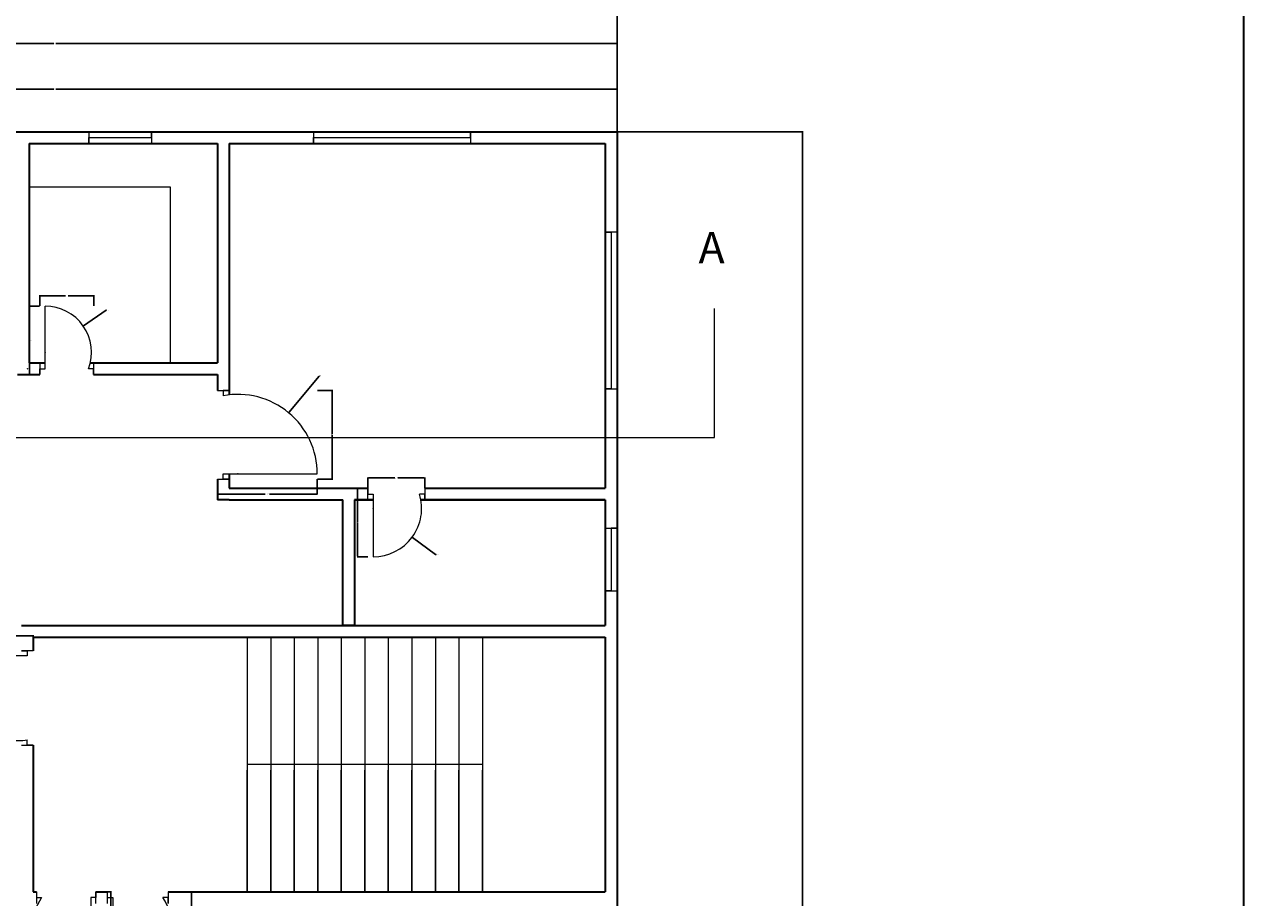
# Model space of a CAD drawing. Units: inches. Extents: x 992 to 2287, y 1476 to 2866.
# Tile 7 of 9: x 1821 to 2287, y 1987 to 2321. Entities that reach past the tile are written whole.
import ezdxf

# ---------------------------------------------------------------- set-up
doc = ezdxf.new("R2010")
doc.units = ezdxf.units.IN
for name, color, linetype, lineweight in [('A-ANNO-DIMS', 2, 'Continuous', 18), ('A-ANNO-SYMB', 2, 'Continuous', 18), ('A-ANNO-TTLB', 7, 'Continuous', 35), ('A-DOOR', 3, 'Continuous', 18), ('A-FLOR-CASE', 9, 'Continuous', 18), ('A-FLOR-STRS', 7, 'Continuous', 18), ('A-GLAZ', 4, 'Continuous', 18), ('A-WALL', 7, 'Continuous', 35)]:
    doc.layers.add(name, color=color, linetype=linetype, lineweight=lineweight)
doc.styles.get("Standard").update_dxf_attribs({"font": 'arial.ttf'})
doc.dimstyles.get("Standard").update_dxf_attribs({"dimtxt": 0.18, "dimasz": 0.18, "dimexe": 0.18, "dimexo": 0.0625, "dimgap": 0.09, "dimtad": 0, "dimtih": 1, "dimtoh": 1, "dimdec": 4, "dimzin": 0, "dimdsep": 46, "dimtxsty": 'Standard', "dimcen": 0.09, "dimadec": 0, "dimazin": 0, "dimtfac": 1, "dimtdec": 4, "dimtofl": 0, "dimtmove": 0, "dimatfit": 3, "dimfxl": 1, "dimtolj": 1, "dimtzin": 0, "dimarcsym": 0})

# ---------------------------------------------------------------- blocks, each defined once
blk = doc.blocks.new('DOOR-SINGLE-36IN-01')
for p, q in [((36, 34.15), (0, 34.15)), ((38.25, 36.15), (33.75, 36.15)), ((33.75, 36.15), (36, 36.15)), ((36, 36.15), (36, 34.15)), ((33.75, 0), (38.25, 0)), ((36, 0), (36, 2)), ((38.25, 0), (36, 0))]:
    blk.add_line(p, q)
blk.add_arc((32.36, 34.15), 32.36, 180, 276.4675)
blk = doc.blocks.new('DOOR-SINGLE-36IN-02')
for p, q in [((0, 33.92), (4.5, 33.92)), ((4.5, 33.92), (2.25, 33.92)), ((2.25, 33.92), (2.25, 31.92)), ((0, 0), (4.5, 0)), ((2.25, 0), (2.25, 2)), ((2.25, 2), (38.25, 2)), ((4.5, 0), (2.25, 0))]:
    blk.add_line(p, q)
blk.add_arc((7.81, 2), 30.44, 0, 100.535)
blk = doc.blocks.new('DOOR-SINGLE-24IN-03')
for p, q in [((0, 21.75), (0, 26.25)), ((0, 26.25), (0, 24)), ((0, 24), (0, 24)), ((0, 24), (2, 24)), ((2, 24), (2, 0)), ((21.76, 24), (19.76, 24)), ((21.76, 26.25), (21.76, 21.75)), ((21.76, 21.75), (21.76, 24))]:
    blk.add_line(p, q)
blk.add_arc((2, 18.57), 18.57, 270, 16.9925)
blk = doc.blocks.new('DOOR-SINGLE-24IN-05')
for p, q in [((2, 2.25), (2, 26.25)), ((0, 4.5), (0, 0)), ((0, 0), (0, 2.25)), ((0, 2.25), (2, 2.25)), ((20.6, 2.25), (18.6, 2.25)), ((20.6, 4.5), (20.6, 0)), ((20.6, 0), (20.6, 2.25))]:
    blk.add_line(p, q)
blk.add_arc((2, 8.51), 17.74, 339.3303, 90)
blk = doc.blocks.new('DOOR-SINGLE-36IN-07')
for p, q in [((2.12, 38.25), (2.12, 33.75)), ((24.9, 33.75), (24.9, 38.25)), ((24.9, 38.25), (24.9, 36)), ((2.12, 36), (4.12, 36)), ((24.9, 36), (22.9, 36)), ((22.9, 36), (22.9, 0))]:
    blk.add_line(p, q)
blk.add_arc((22.9, 22.9), 22.9, 145.0915, 270)
blk = doc.blocks.new('DOOR-SINGLE-36IN-08')
for p, q in [((0, 33.75), (0, 38.25)), ((23.12, 38.25), (23.12, 33.75)), ((0, 36), (2, 36)), ((2, 36), (2, 0)), ((23.12, 36), (21.12, 36)), ((23.12, 33.75), (23.12, 36))]:
    blk.add_line(p, q)
blk.add_arc((2, 23.08), 23.08, 270, 34.0417)
blk = doc.blocks.new('WINDOW-24IN-A')
for p, q in [((0, 24), (4.5, 24)), ((4.5, 24), (2.25, 24)), ((2.25, 24), (2.25, 0)), ((2.25, 0), (0, 0)), ((0, 0), (4.5, 0))]:
    blk.add_line(p, q)
blk = doc.blocks.new('WINDOW-60IN-A')
for p, q in [((4.5, 60), (0, 60)), ((0, 60), (2.25, 60)), ((2.25, 60), (2.25, 0)), ((2.25, 0), (0, 0)), ((0, 0), (4.5, 0))]:
    blk.add_line(p, q)
blk = doc.blocks.new('WINDOW-60IN-B')
for p, q in [((0, 4.5), (0, 0)), ((0, 0), (0, 2.25)), ((0, 2.25), (60, 2.25)), ((60, 2.25), (60, 4.5)), ((60, 4.5), (60, 0))]:
    blk.add_line(p, q)
blk = doc.blocks.new('WINDOW-24IN-B')
for p, q in [((0, 4.5), (0, 4.5)), ((0, 4.5), (0, 0)), ((0, 0), (0, 2.25)), ((0, 2.25), (24, 2.25)), ((24, 2.25), (24, 4.5)), ((24, 4.5), (24, 0))]:
    blk.add_line(p, q)
blk = doc.blocks.new('STAIR-RETURN-PLAN')
for p, q in [((0, 97.5), (0, 0)), ((9, 97.5), (9, 0)), ((18, 97.5), (18, 0)), ((27, 97.5), (27, 0)), ((36, 97.5), (36, 0)), ((45, 97.5), (45, 0)), ((54, 97.5), (54, 0)), ((63, 97.5), (63, 0)), ((72, 97.5), (72, 0)), ((81, 97.5), (81, 0)), ((90, 97.5), (90, 0)), ((90, 48.75), (0, 48.75)), ((0, 0), (0, 46.5)), ((9, 0), (9, 46.5)), ((18, 0), (18, 46.5)), ((27, 0), (27, 46.5)), ((36, 0), (36, 46.5)), ((45, 0), (45, 46.5)), ((54, 0), (54, 46.5)), ((63, 0), (63, 46.5)), ((72, 0), (72, 46.5)), ((81, 0), (81, 46.5)), ((90, 0), (90, 46.5))]:
    blk.add_line(p, q)
blk = doc.blocks.new('COUNTER-L-NORTH')
for p, q in [((0, 67.36), (53.88, 67.36)), ((53.88, 67.36), (53.88, 0))]:
    blk.add_line(p, q)
blk = doc.blocks.new('*D49')
at = {"layer": 'A-ANNO-DIMS', "color": 0, "lineweight": -2, "transparency": 16777216}
for p, q in [((1785.64, 2081.37), (1785.64, 2087.23)), ((1785.82, 2087.05), (1803.98, 2087.05)), ((1823.71, 2087.05), (1805.56, 2087.05)), ((1823.89, 2081.37), (1823.89, 2087.23))]:
    blk.add_line(p, q, dxfattribs=at)
at = {"layer": 'A-ANNO-DIMS', "color": 0, "transparency": 16777216}
for points in [[(1785.82, 2087.08), (1785.82, 2087.02), (1785.64, 2087.05)], [(1823.71, 2087.08), (1823.71, 2087.02), (1823.89, 2087.05)]]:
    blk.add_solid(points, dxfattribs=at)
at = {"layer": 'Defpoints', "color": 0, "transparency": 16777216}
for p in [(1823.89, 2087.05), (1785.64, 2081.31), (1823.89, 2081.31)]:
    blk.add_point(p, dxfattribs=at)
at = {"layer": 'A-ANNO-DIMS', "color": 0, "transparency": 16777216, "insert": (1804.77, 2087.05), "char_height": 0.18, "attachment_point": 5}
blk.add_mtext('\\A1;D01 38 TYP.', dxfattribs=at)
blk = doc.blocks.new('*D51')
at = {"layer": 'A-ANNO-DIMS', "color": 0, "lineweight": -2, "transparency": 16777216}
for p, q in [((1894.39, 2146.99), (1894.39, 2141.13)), ((1932.64, 2146.99), (1932.64, 2141.13)), ((1894.57, 2141.31), (1912.73, 2141.31)), ((1932.46, 2141.31), (1914.31, 2141.31))]:
    blk.add_line(p, q, dxfattribs=at)
at = {"layer": 'A-ANNO-DIMS', "color": 0, "transparency": 16777216}
for points in [[(1894.57, 2141.34), (1894.57, 2141.28), (1894.39, 2141.31)], [(1932.46, 2141.34), (1932.46, 2141.28), (1932.64, 2141.31)]]:
    blk.add_solid(points, dxfattribs=at)
at = {"layer": 'Defpoints', "color": 0, "transparency": 16777216}
for p in [(1894.39, 2147.05), (1932.64, 2147.05), (1932.64, 2141.31)]:
    blk.add_point(p, dxfattribs=at)
at = {"layer": 'A-ANNO-DIMS', "color": 0, "transparency": 16777216, "insert": (1913.52, 2141.31), "char_height": 0.18, "attachment_point": 5}
blk.add_mtext('\\A1;D02 38 TYP.', dxfattribs=at)
blk = doc.blocks.new('*D52')
at = {"layer": 'A-ANNO-DIMS', "color": 0, "lineweight": -2, "transparency": 16777216}
for p, q in [((1932.71, 2180.97), (1938.56, 2180.97)), ((1938.38, 2180.79), (1938.38, 2164.19)), ((1938.38, 2147.23), (1938.38, 2163.83)), ((1932.71, 2147.05), (1938.56, 2147.05))]:
    blk.add_line(p, q, dxfattribs=at)
at = {"layer": 'A-ANNO-DIMS', "color": 0, "transparency": 16777216}
for points in [[(1938.35, 2180.79), (1938.41, 2180.79), (1938.38, 2180.97)], [(1938.35, 2147.23), (1938.41, 2147.23), (1938.38, 2147.05)]]:
    blk.add_solid(points, dxfattribs=at)
at = {"layer": 'Defpoints', "color": 0, "transparency": 16777216}
for p in [(1932.64, 2180.97), (1938.38, 2180.97), (1932.64, 2147.05)]:
    blk.add_point(p, dxfattribs=at)
at = {"layer": 'A-ANNO-DIMS', "color": 0, "transparency": 16777216, "insert": (1938.38, 2164.01), "char_height": 0.18, "attachment_point": 5}
blk.add_mtext('\\A1;34 TYP.', dxfattribs=at)
blk = doc.blocks.new('*D53')
at = {"layer": 'A-ANNO-DIMS', "color": 0, "lineweight": -2, "transparency": 16777216}
for p, q in [((1951.96, 2143.54), (1947.9, 2143.54)), ((1948.08, 2143.36), (1948.08, 2130.6)), ((1948.08, 2117.47), (1948.08, 2130.24)), ((1951.96, 2117.29), (1947.9, 2117.29))]:
    blk.add_line(p, q, dxfattribs=at)
at = {"layer": 'A-ANNO-DIMS', "color": 0, "transparency": 16777216}
for points in [[(1948.05, 2143.36), (1948.11, 2143.36), (1948.08, 2143.54)], [(1948.05, 2117.47), (1948.11, 2117.47), (1948.08, 2117.29)]]:
    blk.add_solid(points, dxfattribs=at)
at = {"layer": 'Defpoints', "color": 0, "transparency": 16777216}
for p in [(1948.08, 2143.54), (1952.02, 2143.54), (1952.02, 2117.29)]:
    blk.add_point(p, dxfattribs=at)
at = {"layer": 'A-ANNO-DIMS', "color": 0, "transparency": 16777216, "insert": (1948.08, 2130.42), "char_height": 0.18, "attachment_point": 5}
blk.add_mtext('\\A1;D03 26 TYP.', dxfattribs=at)
blk = doc.blocks.new('*D54')
at = {"layer": 'A-ANNO-DIMS', "color": 0, "lineweight": -2, "transparency": 16777216}
for p, q in [((1952.02, 2143.61), (1952.02, 2147.66)), ((1952.2, 2147.48), (1962.37, 2147.48)), ((1973.6, 2147.48), (1963.43, 2147.48)), ((1973.78, 2143.61), (1973.78, 2147.66))]:
    blk.add_line(p, q, dxfattribs=at)
at = {"layer": 'A-ANNO-DIMS', "color": 0, "transparency": 16777216}
for points in [[(1952.2, 2147.51), (1952.2, 2147.45), (1952.02, 2147.48)], [(1973.6, 2147.51), (1973.6, 2147.45), (1973.78, 2147.48)]]:
    blk.add_solid(points, dxfattribs=at)
at = {"layer": 'Defpoints', "color": 0, "transparency": 16777216}
for p in [(1973.78, 2147.48), (1952.02, 2143.54), (1973.78, 2143.54)]:
    blk.add_point(p, dxfattribs=at)
at = {"layer": 'A-ANNO-DIMS', "color": 0, "transparency": 16777216, "insert": (1962.9, 2147.48), "char_height": 0.18, "attachment_point": 5}
blk.add_mtext('\\A1;22 TYP.', dxfattribs=at)
blk = doc.blocks.new('*D57')
at = {"layer": 'A-ANNO-DIMS', "color": 0, "lineweight": -2, "transparency": 16777216}
for p, q in [((1826.37, 2213.29), (1822.31, 2213.29)), ((1822.49, 2213.11), (1822.49, 2200.35)), ((1822.49, 2187.22), (1822.49, 2199.99)), ((1826.37, 2187.04), (1822.31, 2187.04))]:
    blk.add_line(p, q, dxfattribs=at)
at = {"layer": 'A-ANNO-DIMS', "color": 0, "transparency": 16777216}
for points in [[(1822.46, 2213.11), (1822.52, 2213.11), (1822.49, 2213.29)], [(1822.46, 2187.22), (1822.52, 2187.22), (1822.49, 2187.04)]]:
    blk.add_solid(points, dxfattribs=at)
at = {"layer": 'Defpoints', "color": 0, "transparency": 16777216}
for p in [(1822.49, 2213.29), (1826.43, 2213.29), (1826.43, 2187.04)]:
    blk.add_point(p, dxfattribs=at)
at = {"layer": 'A-ANNO-DIMS', "color": 0, "transparency": 16777216, "insert": (1822.49, 2200.17), "char_height": 0.18, "attachment_point": 5}
blk.add_mtext('\\A1;D05 26 TYP.', dxfattribs=at)
blk = doc.blocks.new('*D58')
at = {"layer": 'A-ANNO-DIMS', "color": 0, "lineweight": -2, "transparency": 16777216}
for p, q in [((1826.43, 2213.36), (1826.43, 2217.41)), ((1826.61, 2217.23), (1836.23, 2217.23)), ((1846.9, 2217.23), (1837.29, 2217.23)), ((1847.08, 2213.36), (1847.08, 2217.41))]:
    blk.add_line(p, q, dxfattribs=at)
at = {"layer": 'A-ANNO-DIMS', "color": 0, "transparency": 16777216}
for points in [[(1826.61, 2217.26), (1826.61, 2217.2), (1826.43, 2217.23)], [(1846.9, 2217.26), (1846.9, 2217.2), (1847.08, 2217.23)]]:
    blk.add_solid(points, dxfattribs=at)
at = {"layer": 'Defpoints', "color": 0, "transparency": 16777216}
for p in [(1847.08, 2217.23), (1826.43, 2213.29), (1847.08, 2213.29)]:
    blk.add_point(p, dxfattribs=at)
at = {"layer": 'A-ANNO-DIMS', "color": 0, "transparency": 16777216, "insert": (1836.76, 2217.23), "char_height": 0.18, "attachment_point": 5}
blk.add_mtext('\\A1;21 TYP.', dxfattribs=at)
blk = doc.blocks.new('*D61')
at = {"layer": 'A-ANNO-DIMS', "color": 0, "lineweight": -2, "transparency": 16777216}
for p, q in [((1847.96, 1989.04), (1853.81, 1989.04)), ((1853.63, 1988.86), (1853.63, 1970.1)), ((1853.63, 1950.97), (1853.63, 1969.74)), ((1847.96, 1950.79), (1853.81, 1950.79))]:
    blk.add_line(p, q, dxfattribs=at)
at = {"layer": 'A-ANNO-DIMS', "color": 0, "transparency": 16777216}
for points in [[(1853.6, 1988.86), (1853.66, 1988.86), (1853.63, 1989.04)], [(1853.6, 1950.97), (1853.66, 1950.97), (1853.63, 1950.79)]]:
    blk.add_solid(points, dxfattribs=at)
at = {"layer": 'Defpoints', "color": 0, "transparency": 16777216}
for p in [(1847.89, 1989.04), (1853.63, 1989.04), (1847.89, 1950.79)]:
    blk.add_point(p, dxfattribs=at)
at = {"layer": 'A-ANNO-DIMS', "color": 0, "transparency": 16777216, "insert": (1853.63, 1969.92), "char_height": 0.18, "attachment_point": 5}
blk.add_mtext('\\A1;D07 38 TYP.', dxfattribs=at)
blk = doc.blocks.new('*D63')
at = {"layer": 'A-ANNO-DIMS', "color": 0, "lineweight": -2, "transparency": 16777216}
for p, q in [((1878.84, 1989.04), (1884.7, 1989.04)), ((1884.52, 1988.86), (1884.52, 1970.1)), ((1884.52, 1950.97), (1884.52, 1969.74)), ((1878.84, 1950.79), (1884.7, 1950.79))]:
    blk.add_line(p, q, dxfattribs=at)
at = {"layer": 'A-ANNO-DIMS', "color": 0, "transparency": 16777216}
for points in [[(1884.49, 1988.86), (1884.55, 1988.86), (1884.52, 1989.04)], [(1884.49, 1950.97), (1884.55, 1950.97), (1884.52, 1950.79)]]:
    blk.add_solid(points, dxfattribs=at)
at = {"layer": 'Defpoints', "color": 0, "transparency": 16777216}
for p in [(1878.78, 1989.04), (1884.52, 1989.04), (1878.78, 1950.79)]:
    blk.add_point(p, dxfattribs=at)
at = {"layer": 'A-ANNO-DIMS', "color": 0, "transparency": 16777216, "insert": (1884.52, 1969.92), "char_height": 0.18, "attachment_point": 5}
blk.add_mtext('\\A1;D08 38 TYP.', dxfattribs=at)
blk = doc.blocks.new('*D111')
at = {"layer": 'A-ANNO-DIMS', "color": 0, "lineweight": -2, "transparency": 16777216}
for p, q in [((1616.89, 2280.11), (1616.89, 2314.02)), ((1617.07, 2313.84), (1831.75, 2313.84)), ((2047.21, 2313.84), (1832.54, 2313.84)), ((2047.39, 2280.11), (2047.39, 2314.02))]:
    blk.add_line(p, q, dxfattribs=at)
at = {"layer": 'A-ANNO-DIMS', "color": 0, "transparency": 16777216}
for points in [[(1617.07, 2313.87), (1617.07, 2313.81), (1616.89, 2313.84)], [(2047.21, 2313.87), (2047.21, 2313.81), (2047.39, 2313.84)]]:
    blk.add_solid(points, dxfattribs=at)
at = {"layer": 'Defpoints', "color": 0, "transparency": 16777216}
for p in [(2047.39, 2313.84), (1616.89, 2280.04), (2047.39, 2280.04)]:
    blk.add_point(p, dxfattribs=at)
at = {"layer": 'A-ANNO-DIMS', "color": 0, "transparency": 16777216, "insert": (1832.14, 2313.84), "char_height": 0.18, "attachment_point": 5}
blk.add_mtext('\\A1;430.5', dxfattribs=at)
blk = doc.blocks.new('*D112')
at = {"layer": 'A-ANNO-DIMS', "color": 0, "lineweight": -2, "transparency": 16777216}
for p, q in [((2047.46, 2280.04), (2118.61, 2280.04)), ((2118.43, 2279.86), (2118.43, 1955.47)), ((2118.43, 1630.72), (2118.43, 1955.11)), ((2047.46, 1630.54), (2118.61, 1630.54))]:
    blk.add_line(p, q, dxfattribs=at)
at = {"layer": 'A-ANNO-DIMS', "color": 0, "transparency": 16777216}
for points in [[(2118.4, 2279.86), (2118.46, 2279.86), (2118.43, 2280.04)], [(2118.4, 1630.72), (2118.46, 1630.72), (2118.43, 1630.54)]]:
    blk.add_solid(points, dxfattribs=at)
at = {"layer": 'Defpoints', "color": 0, "transparency": 16777216}
for p in [(2047.39, 2280.04), (2118.43, 2280.04), (2047.39, 1630.54)]:
    blk.add_point(p, dxfattribs=at)
at = {"layer": 'A-ANNO-DIMS', "color": 0, "transparency": 16777216, "insert": (2118.43, 1955.29), "char_height": 0.18, "attachment_point": 5}
blk.add_mtext('\\A1;649.5', dxfattribs=at)
blk = doc.blocks.new('*D142')
at = {"layer": 'A-ANNO-DIMS', "color": 0, "lineweight": -2, "transparency": 16777216}
for p, q in [((1616.89, 2366.07), (1616.89, 2296.22)), ((2047.39, 2366.07), (2047.39, 2296.22)), ((1617.07, 2296.4), (1831.75, 2296.4)), ((2047.21, 2296.4), (1832.54, 2296.4))]:
    blk.add_line(p, q, dxfattribs=at)
at = {"layer": 'A-ANNO-DIMS', "color": 0, "transparency": 16777216}
for points in [[(1617.07, 2296.43), (1617.07, 2296.37), (1616.89, 2296.4)], [(2047.21, 2296.43), (2047.21, 2296.37), (2047.39, 2296.4)]]:
    blk.add_solid(points, dxfattribs=at)
at = {"layer": 'Defpoints', "color": 0, "transparency": 16777216}
for p in [(1616.89, 2366.13), (2047.39, 2366.13), (2047.39, 2296.4)]:
    blk.add_point(p, dxfattribs=at)
at = {"layer": 'A-ANNO-DIMS', "color": 0, "transparency": 16777216, "insert": (1832.14, 2296.4), "char_height": 0.18, "attachment_point": 5}
blk.add_mtext('\\A1;430.5', dxfattribs=at)
blk = doc.blocks.new('*D154')
at = {"layer": 'A-ANNO-DIMS', "color": 0, "lineweight": -2, "transparency": 16777216}
for p, q in [((1933.34, 2186.5), (1921.78, 2172.59)), ((1933.52, 2186.5), (1933.34, 2186.5)), ((1902.12, 2149.05), (1902.3, 2149.05)), ((1902.21, 2148.96), (1902.21, 2149.14))]:
    blk.add_line(p, q, dxfattribs=at)
at = {"layer": 'A-ANNO-DIMS', "color": 0, "transparency": 16777216}
blk.add_solid([(1921.76, 2172.61), (1921.8, 2172.57), (1921.66, 2172.45)], dxfattribs=at)
at = {"layer": 'Defpoints', "color": 0, "transparency": 16777216}
for p in [(1921.66, 2172.45), (1902.21, 2149.05)]:
    blk.add_point(p, dxfattribs=at)
at = {"layer": 'A-ANNO-DIMS', "color": 0, "transparency": 16777216, "insert": (1934.07, 2186.5), "char_height": 0.18, "attachment_point": 5}
blk.add_mtext('\\A1;R30.435', dxfattribs=at)
blk = doc.blocks.new('*D158')
at = {"layer": 'A-ANNO-DIMS', "color": 0, "lineweight": -2, "transparency": 16777216}
for p, q in [((1787.27, 2212.46), (1787.45, 2212.46)), ((1787.45, 2212.46), (1800.17, 2203.87)), ((1821.68, 2189.29), (1821.86, 2189.29)), ((1821.77, 2189.2), (1821.77, 2189.38))]:
    blk.add_line(p, q, dxfattribs=at)
at = {"layer": 'A-ANNO-DIMS', "color": 0, "transparency": 16777216}
blk.add_solid([(1800.19, 2203.9), (1800.16, 2203.85), (1800.32, 2203.77)], dxfattribs=at)
at = {"layer": 'Defpoints', "color": 0, "transparency": 16777216}
for p in [(1800.32, 2203.77), (1821.77, 2189.29)]:
    blk.add_point(p, dxfattribs=at)
at = {"layer": 'A-ANNO-DIMS', "color": 0, "transparency": 16777216, "insert": (1786.79, 2212.46), "char_height": 0.18, "attachment_point": 5}
blk.add_mtext('\\A1;R25.88', dxfattribs=at)
blk = doc.blocks.new('*D165')
at = {"layer": 'A-ANNO-DIMS', "color": 0, "lineweight": -2, "transparency": 16777216}
for p, q in [((1953.93, 2135.87), (1954.11, 2135.87)), ((1954.02, 2135.78), (1954.02, 2135.96)), ((1977.9, 2118.19), (1969.09, 2124.71)), ((1978.08, 2118.19), (1977.9, 2118.19))]:
    blk.add_line(p, q, dxfattribs=at)
at = {"layer": 'A-ANNO-DIMS', "color": 0, "transparency": 16777216}
blk.add_solid([(1969.11, 2124.73), (1969.07, 2124.69), (1968.95, 2124.82)], dxfattribs=at)
at = {"layer": 'Defpoints', "color": 0, "transparency": 16777216}
for p in [(1954.02, 2135.87), (1968.95, 2124.82)]:
    blk.add_point(p, dxfattribs=at)
at = {"layer": 'A-ANNO-DIMS', "color": 0, "transparency": 16777216, "insert": (1978.63, 2118.19), "char_height": 0.18, "attachment_point": 5}
blk.add_mtext('\\A1;R18.572', dxfattribs=at)
blk = doc.blocks.new('*D167')
at = {"layer": 'A-ANNO-DIMS', "color": 0, "lineweight": -2, "transparency": 16777216}
for p, q in [((1851.78, 2211.7), (1843.17, 2205.75)), ((1851.96, 2211.7), (1851.78, 2211.7)), ((1828.34, 2195.55), (1828.52, 2195.55)), ((1828.43, 2195.46), (1828.43, 2195.64))]:
    blk.add_line(p, q, dxfattribs=at)
at = {"layer": 'A-ANNO-DIMS', "color": 0, "transparency": 16777216}
blk.add_solid([(1843.15, 2205.77), (1843.19, 2205.72), (1843.02, 2205.64)], dxfattribs=at)
at = {"layer": 'Defpoints', "color": 0, "transparency": 16777216}
for p in [(1843.02, 2205.64), (1828.43, 2195.55)]:
    blk.add_point(p, dxfattribs=at)
at = {"layer": 'A-ANNO-DIMS', "color": 0, "transparency": 16777216, "insert": (1852.43, 2211.7), "char_height": 0.18, "attachment_point": 5}
blk.add_mtext('\\A1;R17.74', dxfattribs=at)

msp = doc.modelspace()

# ---------------------------------------------------------------- linework, layer by layer
at = {"layer": 'A-ANNO-SYMB'}
for p, q in [((2084.6292, 2162.9718), (2084.6292, 2212.3883)), ((1598.561, 2162.9718), (2084.6292, 2162.9718))]:
    msp.add_line(p, q, dxfattribs=at)
at = {"layer": 'A-ANNO-TTLB'}
msp.add_lwpolyline([(992.3484, 2866.1952), (2287.217, 2866.1952), (2287.217, 1476.4066), (992.3484, 1476.4066)], close=True, dxfattribs=at)
at = {"layer": 'A-WALL'}
for p, q in [((1616.8946, 2280.0428), (2047.3946, 2280.0428)), ((1616.8946, 2280.0428), (2047.3946, 2280.0428)), ((2047.3946, 2280.0428), (2047.3946, 1677.0428)), ((1822.3946, 2275.5428), (1894.3946, 2275.5428)), ((1822.3946, 2275.5428), (1822.3946, 2191.5428)), ((1894.3946, 2275.5428), (1894.3946, 2191.5428)), ((1898.8946, 2275.5428), (2042.8946, 2275.5428)), ((1898.8946, 2275.5428), (1898.8946, 2179.3035)), ((2042.8946, 2275.5428), (2042.8946, 2143.5428)), ((1822.3946, 2191.5428), (1828.4319, 2191.5428)), ((1845.711, 2191.5428), (1894.3946, 2191.5428)), ((1817.8946, 2187.0428), (1826.4319, 2187.0428)), ((1847.0287, 2187.0428), (1894.3946, 2187.0428)), ((1894.3946, 2187.0428), (1894.3946, 2180.9715)), ((1894.3946, 2147.0492), (1894.3946, 2139.0428)), ((1898.8946, 2149.0492), (1898.8946, 2143.5428)), ((1898.8946, 2143.5428), (1952.0185, 2143.5428)), ((1973.78, 2143.5428), (2042.8946, 2143.5428)), ((1898.8946, 2139.0428), (1894.3946, 2139.0428)), ((1898.8946, 2139.0428), (1942.3946, 2139.0428)), ((1942.3946, 2091.0428), (1942.3946, 2139.0428)), ((1946.8946, 2139.0428), (1954.0185, 2139.0428)), ((1954.0185, 2139.0428), (1946.8946, 2139.0428)), ((1946.8946, 2139.0428), (1946.8946, 2091.0428)), ((1972.317, 2139.0428), (2042.8946, 2139.0428)), ((2042.8946, 2139.0428), (1972.317, 2139.0428)), ((2042.8946, 2139.0428), (2042.8946, 2091.0428)), ((1819.3946, 2091.0428), (2042.8946, 2091.0428)), ((1946.8946, 2091.0428), (1942.3946, 2091.0428)), ((1823.8946, 2086.5428), (2042.8946, 2086.5428)), ((1823.8946, 2086.5428), (1823.8946, 2081.3118)), ((2042.8946, 2086.5428), (2042.8946, 1989.0428)), ((1823.8946, 2045.1622), (1823.8946, 1989.0428)), ((1823.8946, 1989.0428), (1825.1176, 1989.0428)), ((1847.8946, 1989.0428), (1852.3946, 1989.0428)), ((1875.5193, 1989.0428), (2042.8946, 1989.0428)), ((2047.3946, 1989.0428), (2047.3946, 1984.5428))]:
    msp.add_line(p, q, dxfattribs=at)

# ---------------------------------------------------------------- block references
at = {"layer": 'A-DOOR'}
for name, p in [('DOOR-SINGLE-24IN-05', (1826.432, 2187.043)), ('DOOR-SINGLE-36IN-02', (1894.395, 2147.049)), ('DOOR-SINGLE-24IN-03', (1952.018, 2117.293)), ('DOOR-SINGLE-36IN-01', (1785.645, 2045.162)), ('DOOR-SINGLE-36IN-07', (1822.998, 1950.793)), ('DOOR-SINGLE-36IN-08', (1852.395, 1950.793))]:
    msp.add_blockref(name, p, dxfattribs=at)
at = {"layer": 'A-FLOR-CASE'}
msp.add_blockref('COUNTER-L-NORTH', (1822.395, 2191.543), dxfattribs=at)
at = {"layer": 'A-FLOR-STRS'}
msp.add_blockref('STAIR-RETURN-PLAN', (1905.828, 1989.043), dxfattribs=at)
at = {"layer": 'A-GLAZ'}
for name, p in [('WINDOW-24IN-B', (1845.184, 2275.543)), ('WINDOW-60IN-B', (1931.223, 2275.543)), ('WINDOW-60IN-A', (2042.895, 2181.633)), ('WINDOW-24IN-A', (2042.895, 2104.303))]:
    msp.add_blockref(name, p, dxfattribs=at)

# ---------------------------------------------------------------- texts
at = {"layer": 'A-ANNO-SYMB', "insert": (2078.6017, 2241.6867), "char_height": 12, "attachment_point": 1}
msp.add_mtext_dynamic_manual_height_columns('A', width=37.726322, gutter_width=12.5, heights=[0], dxfattribs=at)

# ---------------------------------------------------------------- dimensions: what is measured, and where the dimension line sits
at = {"layer": 'A-ANNO-DIMS'}
for base, p1, p2, picture, middle in [((2047.3946, 2296.4015), (1616.8946, 2366.1302), (2047.3946, 2366.1302), '*D142', (1832.1446, 2296.4015)), ((2047.3946, 2313.8428), (1616.8946, 2280.0428), (2047.3946, 2280.0428), '*D111', (1832.1446, 2313.8428))]:
    dim = msp.add_linear_dim(base=base, p1=p1, p2=p2, dimstyle='Standard', override={"dimdec": 1, "dimlfac": 1, "dimrnd": 0, "dimzin": 0, "dimdsep": 46, "dimlunit": 2}, dxfattribs=at)
    dim.commit()
    dim.dimension.update_dxf_attribs({"geometry": picture, "text_midpoint": middle})
dim = msp.add_linear_dim(base=(2118.4292, 2280.0428), p1=(2047.3946, 1630.5428), p2=(2047.3946, 2280.0428), angle=90, dimstyle='Standard', override={"dimdec": 1, "dimlfac": 1, "dimrnd": 0, "dimzin": 0, "dimdsep": 46, "dimlunit": 2}, dxfattribs=at)
dim.commit()
dim.dimension.update_dxf_attribs({"geometry": '*D112', "text_midpoint": (2118.4292, 1955.2928)})
for base, p1, p2, text, picture, middle in [((1847.0845, 2217.2303), (1826.4319, 2213.2928), (1847.0845, 2213.2928), '<> TYP.', '*D58', (1836.7582, 2217.2303)), ((1932.6446, 2141.3117), (1894.3946, 2147.0492), (1932.6446, 2147.0492), 'D02 <> TYP.', '*D51', (1913.5196, 2141.3117)), ((1973.78, 2147.4803), (1952.0185, 2143.5428), (1973.78, 2143.5428), '<> TYP.', '*D54', (1962.8993, 2147.4803)), ((1823.8946, 2087.0493), (1785.6446, 2081.3118), (1823.8946, 2081.3118), 'D01 <> TYP.', '*D49', (1804.7696, 2087.0493))]:
    dim = msp.add_linear_dim(base=base, p1=p1, p2=p2, text=text, dimstyle='Standard', override={"dimdec": 0, "dimlfac": 1, "dimrnd": 0, "dimzin": 0, "dimdsep": 46, "dimlunit": 2}, dxfattribs=at)
    dim.commit()
    dim.dimension.update_dxf_attribs({"geometry": picture, "text_midpoint": middle})
for center, mpoint, override, picture, middle in [((1821.7729, 2189.2928), (1800.323, 2203.77), {"dimdec": 2, "dimlfac": 1, "dimrnd": 0, "dimzin": 0, "dimdsep": 46, "dimlunit": 2}, '*D158', (1786.7931, 2212.4563)), ((1828.4319, 2195.5542), (1843.0216, 2205.6437), {"dimdec": 2, "dimlfac": 1, "dimrnd": 0, "dimzin": 0, "dimdsep": 46, "dimlunit": 2}, '*D167', (1852.4349, 2211.6974)), ((1902.2093, 2149.0492), (1921.6639, 2172.4549), {"dimdec": 3, "dimlfac": 1, "dimrnd": 0, "dimzin": 0, "dimdsep": 46, "dimlunit": 2}, '*D154', (1934.0672, 2186.4983)), ((1954.0185, 2135.8651), (1968.9472, 2124.8168), {"dimdec": 3, "dimlfac": 1, "dimrnd": 0, "dimzin": 0, "dimdsep": 46, "dimlunit": 2}, '*D165', (1978.6333, 2118.1879))]:
    dim = msp.add_radius_dim(center=center, mpoint=mpoint, dimstyle='Standard', override=override, dxfattribs=at)
    dim.commit()
    dim.dimension.update_dxf_attribs({"geometry": picture, "text_midpoint": middle, "dimtype": 164})
for base, p1, p2, text, picture, middle in [((1822.4944, 2213.2928), (1826.4319, 2187.0428), (1826.4319, 2213.2928), 'D05 <> TYP.', '*D57', (1822.4944, 2200.1678)), ((1938.3821, 2180.9715), (1932.6446, 2147.0492), (1932.6446, 2180.9715), '<> TYP.', '*D52', (1938.3821, 2164.0104)), ((1948.081, 2143.5428), (1952.0185, 2117.2928), (1952.0185, 2143.5428), 'D03 <> TYP.', '*D53', (1948.081, 2130.4178)), ((1853.6321, 1989.0428), (1847.8946, 1950.7928), (1847.8946, 1989.0428), 'D07 <> TYP.', '*D61', (1853.6321, 1969.9178)), ((1884.5196, 1989.0428), (1878.7821, 1950.7928), (1878.7821, 1989.0428), 'D08 <> TYP.', '*D63', (1884.5196, 1969.9178))]:
    dim = msp.add_linear_dim(base=base, p1=p1, p2=p2, angle=90, text=text, dimstyle='Standard', override={"dimdec": 0, "dimlfac": 1, "dimrnd": 0, "dimzin": 0, "dimdsep": 46, "dimlunit": 2}, dxfattribs=at)
    dim.commit()
    dim.dimension.update_dxf_attribs({"geometry": picture, "text_midpoint": middle})

doc.saveas('drawing.dxf')
